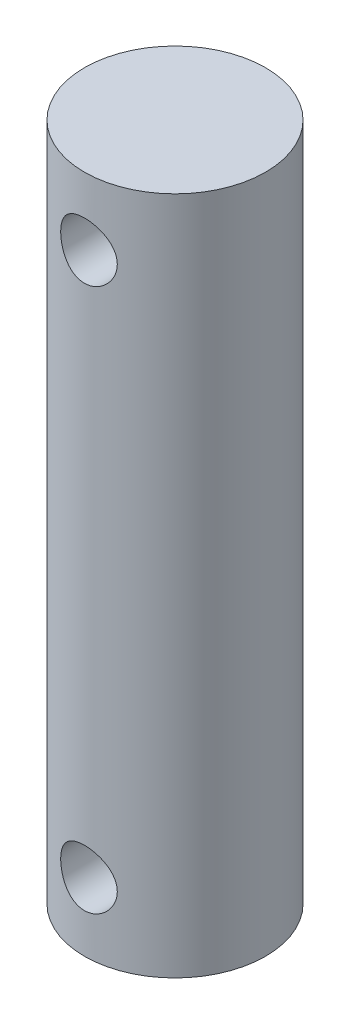
SolidWorks part; units mm, degrees
material "Plain Carbon Steel"
ref_plane "Front Plane" through (0, 0, 0) normal (0, 0, 1) x (1, 0, 0)
ref_plane "Top Plane" through (0, 0, 0) normal (0, 1, 0) x (1, 0, 0)
ref_plane "Right Plane" through (0, 0, 0) normal (1, 0, 0) x (0, 0, -1)
sketch "Pin Profile Ø16" plane through (0, 0, 0) normal (0, 1, 0) x (1, 0, 0)
  circle A0 centre (0, 0) radius 8
  dimension "D1" = 16
extrude "Pin Body Ø16x60" add sketch "Pin Profile Ø16" along normal mid plane 60
sketch "Cross Hole Profile" plane through (0, 0, 0) normal (0, 0, 1) x (1, 0, 0)
  line L0 (8, 30) -> (-8, 30) construction
  line L1 (0, 0) -> (18.6394, 0) construction
  circle A0 centre (0, 24) radius 2.5
  circle A1 centre (0, -24) radius 2.5
  dimension "D1" = 5
  dimension "D2" = 6
extrude "Cross Holes" cut sketch "Cross Hole Profile" against normal through all both and the other way through all
